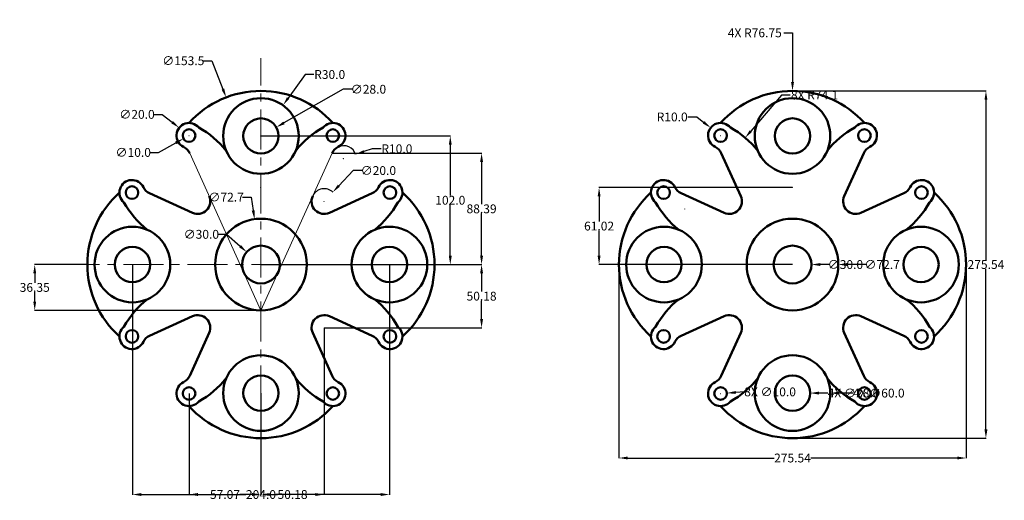
# Model space of a CAD drawing. Units: millimetres. Extents: x -118 to 663, y -125 to 257.
import ezdxf

# ---------------------------------------------------------------- set-up
doc = ezdxf.new("R2010")
doc.units = ezdxf.units.MM
doc.header["$MEASUREMENT"] = 0
doc.linetypes.add('CENTER', pattern=[50.8, 31.75, -6.35, 6.35, -6.35])
for name, color, linetype, lineweight in [('M-CNTR', 1, 'CENTER', 18), ('M-CONS', 8, 'Continuous', 13), ('M-DIMS', 3, 'Continuous', 25), ('M-OUTL', 7, 'Continuous', 50)]:
    doc.layers.add(name, color=color, linetype=linetype, lineweight=lineweight)
doc.styles.get("Standard").update_dxf_attribs({"font": 'arial.ttf'})
doc.dimstyles.get("Standard").update_dxf_attribs({"dimtxt": 7, "dimasz": 7, "dimexe": 0.18, "dimexo": 0.0625, "dimgap": 0.09, "dimtad": 0, "dimtih": 1, "dimtoh": 1, "dimdec": 1, "dimzin": 0, "dimdsep": 46, "dimtxsty": 'Standard', "dimcen": 0.09, "dimadec": 0, "dimazin": 0, "dimtfac": 1, "dimtdec": 1, "dimtofl": 0, "dimtmove": 0, "dimatfit": 3, "dimfxl": 1, "dimtolj": 1, "dimtzin": 0, "dimarcsym": 0})

# ---------------------------------------------------------------- blocks, each defined once
blk = doc.blocks.new('*D1')
at = {"layer": 'Defpoints', "color": 0, "transparency": 16777216}
for p in [(73.13, 164.34), (223.4, 164.34), (73.13, 62.34)]:
    blk.add_point(p, dxfattribs=at)
at = {"layer": 'M-DIMS', "color": 0, "lineweight": -2, "transparency": 16777216}
for p, q in [((73.19, 164.34), (223.58, 164.34)), ((223.4, 157.34), (223.4, 117.01)), ((223.4, 69.34), (223.4, 109.68)), ((73.19, 62.34), (223.58, 62.34))]:
    blk.add_line(p, q, dxfattribs=at)
at = {"layer": 'M-DIMS', "color": 0, "transparency": 16777216}
for points in [[(222.24, 157.34), (224.57, 157.34), (223.4, 164.34)], [(222.24, 69.34), (224.57, 69.34), (223.4, 62.34)]]:
    blk.add_solid(points, dxfattribs=at)
at = {"layer": 'M-DIMS', "color": 0, "transparency": 16777216, "insert": (223.4, 113.34), "char_height": 7, "attachment_point": 5}
blk.add_mtext('\\A1;102.0', dxfattribs=at)
blk = doc.blocks.new('*D2')
at = {"layer": 'Defpoints', "color": 0, "transparency": 16777216}
for p in [(130.17, 119.79), (116.43, 105.25)]:
    blk.add_point(p, dxfattribs=at)
at = {"layer": 'M-DIMS', "color": 0, "lineweight": -2, "transparency": 16777216}
for p, q in [((146.36, 136.91), (134.98, 124.87)), ((153.36, 136.91), (146.36, 136.91)), ((123.21, 112.52), (123.39, 112.52)), ((123.3, 112.43), (123.3, 112.61))]:
    blk.add_line(p, q, dxfattribs=at)
blk.add_arc((123.3, 112.52), 10, 45.57695, 155.27019, dxfattribs=at)
at = {"layer": 'M-DIMS', "color": 0, "transparency": 16777216}
blk.add_solid([(134.14, 125.67), (135.83, 124.07), (130.17, 119.79)], dxfattribs=at)
at = {"layer": 'M-DIMS', "color": 0, "transparency": 16777216, "insert": (166.34, 136.91), "char_height": 7, "attachment_point": 5}
blk.add_mtext('\\A1;∅20.0', dxfattribs=at)
blk = doc.blocks.new('*D3')
at = {"layer": 'Defpoints', "color": 0, "transparency": 16777216}
for p in [(61.85, 72.23), (84.4, 52.45)]:
    blk.add_point(p, dxfattribs=at)
at = {"layer": 'M-DIMS', "color": 0, "lineweight": -2, "transparency": 16777216}
for p, q in [((38.8, 86.31), (45.8, 86.31)), ((45.8, 86.31), (56.59, 76.85)), ((73.04, 62.34), (73.22, 62.34)), ((73.13, 62.25), (73.13, 62.43))]:
    blk.add_line(p, q, dxfattribs=at)
at = {"layer": 'M-DIMS', "color": 0, "transparency": 16777216}
blk.add_solid([(57.36, 77.73), (55.82, 75.97), (61.85, 72.23)], dxfattribs=at)
at = {"layer": 'M-DIMS', "color": 0, "transparency": 16777216, "insert": (25.82, 86.31), "char_height": 7, "attachment_point": 5}
blk.add_mtext('\\A1;∅30.0', dxfattribs=at)
blk = doc.blocks.new('*D4')
at = {"layer": 'Defpoints', "color": 0, "transparency": 16777216}
for p in [(67.99, 98.33), (78.26, 26.36)]:
    blk.add_point(p, dxfattribs=at)
at = {"layer": 'M-DIMS', "color": 0, "lineweight": -2, "transparency": 16777216}
for p, q in [((58.49, 115.82), (65.49, 115.82)), ((65.49, 115.82), (67, 105.26)), ((73.04, 62.34), (73.22, 62.34)), ((73.13, 62.25), (73.13, 62.43))]:
    blk.add_line(p, q, dxfattribs=at)
at = {"layer": 'M-DIMS', "color": 0, "transparency": 16777216}
blk.add_solid([(68.16, 105.42), (65.85, 105.09), (67.99, 98.33)], dxfattribs=at)
at = {"layer": 'M-DIMS', "color": 0, "transparency": 16777216, "insert": (45.5, 115.82), "char_height": 7, "attachment_point": 5}
blk.add_mtext('\\A1;∅72.7', dxfattribs=at)
blk = doc.blocks.new('*D5')
at = {"layer": 'Defpoints', "color": 0, "transparency": 16777216}
for p in [(20.44, 167.09), (11.68, 162.27)]:
    blk.add_point(p, dxfattribs=at)
at = {"layer": 'M-DIMS', "color": 0, "lineweight": -2, "transparency": 16777216}
for p, q in [((15.97, 164.68), (16.15, 164.68)), ((16.06, 164.59), (16.06, 164.77)), ((-8.28, 151.29), (5.54, 158.9)), ((-15.28, 151.29), (-8.28, 151.29))]:
    blk.add_line(p, q, dxfattribs=at)
at = {"layer": 'M-DIMS', "color": 0, "transparency": 16777216}
blk.add_solid([(4.98, 159.92), (6.11, 157.88), (11.68, 162.27)], dxfattribs=at)
at = {"layer": 'M-DIMS', "color": 0, "transparency": 16777216, "insert": (-28.26, 151.29), "char_height": 7, "attachment_point": 5}
blk.add_mtext('\\A1;∅10.0', dxfattribs=at)
blk = doc.blocks.new('*D6')
at = {"layer": 'Defpoints', "color": 0, "transparency": 16777216}
for p in [(8.21, 170.87), (23.91, 158.49)]:
    blk.add_point(p, dxfattribs=at)
at = {"layer": 'M-DIMS', "color": 0, "lineweight": -2, "transparency": 16777216}
for p, q in [((-12.26, 181.48), (-5.26, 181.48)), ((-5.26, 181.48), (2.71, 175.2)), ((15.97, 164.68), (16.15, 164.68)), ((16.06, 164.59), (16.06, 164.77))]:
    blk.add_line(p, q, dxfattribs=at)
at = {"layer": 'M-DIMS', "color": 0, "transparency": 16777216}
blk.add_solid([(3.43, 176.12), (1.99, 174.29), (8.21, 170.87)], dxfattribs=at)
at = {"layer": 'M-DIMS', "color": 0, "transparency": 16777216, "insert": (-25.24, 181.48), "char_height": 7, "attachment_point": 5}
blk.add_mtext('\\A1;∅20.0', dxfattribs=at)
blk = doc.blocks.new('*D7')
at = {"layer": 'Defpoints', "color": 0, "transparency": 16777216}
for p in [(85.3, 171.25), (60.95, 157.44)]:
    blk.add_point(p, dxfattribs=at)
at = {"layer": 'M-DIMS', "color": 0, "lineweight": -2, "transparency": 16777216}
for p, q in [((138.48, 201.41), (91.39, 174.7)), ((145.48, 201.41), (138.48, 201.41)), ((73.04, 164.34), (73.22, 164.34)), ((73.13, 164.25), (73.13, 164.43))]:
    blk.add_line(p, q, dxfattribs=at)
at = {"layer": 'M-DIMS', "color": 0, "transparency": 16777216}
blk.add_solid([(90.82, 175.72), (91.97, 173.69), (85.3, 171.25)], dxfattribs=at)
at = {"layer": 'M-DIMS', "color": 0, "transparency": 16777216, "insert": (158.46, 201.41), "char_height": 7, "attachment_point": 5}
blk.add_mtext('\\A1;∅28.0', dxfattribs=at)
blk = doc.blocks.new('*D8')
at = {"layer": 'Defpoints', "color": 0, "transparency": 16777216}
for p in [(90.64, 188.7), (73.13, 164.34)]:
    blk.add_point(p, dxfattribs=at)
at = {"layer": 'M-DIMS', "color": 0, "lineweight": -2, "transparency": 16777216}
for p, q in [((108.18, 213.12), (94.72, 194.39)), ((115.18, 213.12), (108.18, 213.12)), ((73.04, 164.34), (73.22, 164.34)), ((73.13, 164.25), (73.13, 164.43))]:
    blk.add_line(p, q, dxfattribs=at)
at = {"layer": 'M-DIMS', "color": 0, "transparency": 16777216}
blk.add_solid([(93.77, 195.07), (95.67, 193.71), (90.64, 188.7)], dxfattribs=at)
at = {"layer": 'M-DIMS', "color": 0, "transparency": 16777216, "insert": (127.7, 213.12), "char_height": 7, "attachment_point": 5}
blk.add_mtext('\\A1;R30.0', dxfattribs=at)
blk = doc.blocks.new('*D9')
at = {"layer": 'Defpoints', "color": 0, "transparency": 16777216}
for p in [(148.23, 149.76), (138.74, 146.6)]:
    blk.add_point(p, dxfattribs=at)
at = {"layer": 'M-DIMS', "color": 0, "lineweight": -2, "transparency": 16777216}
for p, q in [((161.51, 154.19), (154.87, 151.97)), ((168.51, 154.19), (161.51, 154.19)), ((138.65, 146.6), (138.83, 146.6)), ((138.74, 146.51), (138.74, 146.69))]:
    blk.add_line(p, q, dxfattribs=at)
blk.add_arc((138.74, 146.6), 10, 17.39119, 114.94899, dxfattribs=at)
at = {"layer": 'M-DIMS', "color": 0, "transparency": 16777216}
blk.add_solid([(154.5, 153.08), (155.24, 150.87), (148.23, 149.76)], dxfattribs=at)
at = {"layer": 'M-DIMS', "color": 0, "transparency": 16777216, "insert": (181.03, 154.19), "char_height": 7, "attachment_point": 5}
blk.add_mtext('\\A1;R10.0', dxfattribs=at)
blk = doc.blocks.new('*D10')
at = {"layer": 'Defpoints', "color": 0, "transparency": 16777216}
for p in [(45.48, 194.96), (100.77, 51.76)]:
    blk.add_point(p, dxfattribs=at)
at = {"layer": 'M-DIMS', "color": 0, "lineweight": -2, "transparency": 16777216}
for p, q in [((27.25, 224.05), (34.25, 224.05)), ((34.25, 224.05), (42.96, 201.49)), ((73.04, 123.36), (73.22, 123.36)), ((73.13, 123.27), (73.13, 123.45))]:
    blk.add_line(p, q, dxfattribs=at)
at = {"layer": 'M-DIMS', "color": 0, "transparency": 16777216}
blk.add_solid([(44.05, 201.91), (41.87, 201.07), (45.48, 194.96)], dxfattribs=at)
at = {"layer": 'M-DIMS', "color": 0, "transparency": 16777216, "insert": (11.51, 224.05), "char_height": 7, "attachment_point": 5}
blk.add_mtext('\\A1;∅153.5', dxfattribs=at)
blk = doc.blocks.new('*D11')
at = {"layer": 'Defpoints', "color": 0, "transparency": 16777216}
for p in [(-28.87, 62.34), (175.13, 62.34), (175.13, -120.14)]:
    blk.add_point(p, dxfattribs=at)
at = {"layer": 'M-DIMS', "color": 0, "lineweight": -2, "transparency": 16777216}
for p, q in [((-28.87, 62.28), (-28.87, -120.32)), ((175.13, 62.28), (175.13, -120.32)), ((-21.87, -120.14), (61.18, -120.14)), ((168.13, -120.14), (85.08, -120.14))]:
    blk.add_line(p, q, dxfattribs=at)
at = {"layer": 'M-DIMS', "color": 0, "transparency": 16777216}
for points in [[(-21.87, -118.97), (-21.87, -121.3), (-28.87, -120.14)], [(168.13, -118.97), (168.13, -121.3), (175.13, -120.14)]]:
    blk.add_solid(points, dxfattribs=at)
at = {"layer": 'M-DIMS', "color": 0, "transparency": 16777216, "insert": (73.13, -120.14), "char_height": 7, "attachment_point": 5}
blk.add_mtext('\\A1;204.0', dxfattribs=at)
blk = doc.blocks.new('*D12')
at = {"layer": 'Defpoints', "color": 0, "transparency": 16777216}
for p in [(16.06, -40), (73.13, -39.66), (73.13, -120.14)]:
    blk.add_point(p, dxfattribs=at)
at = {"layer": 'M-DIMS', "color": 0, "lineweight": -2, "transparency": 16777216}
for p, q in [((16.06, -40.06), (16.06, -120.32)), ((73.13, -39.72), (73.13, -120.32)), ((23.06, -120.14), (32.69, -120.14)), ((66.13, -120.14), (56.49, -120.14))]:
    blk.add_line(p, q, dxfattribs=at)
at = {"layer": 'M-DIMS', "color": 0, "transparency": 16777216}
for points in [[(23.06, -118.97), (23.06, -121.3), (16.06, -120.14)], [(66.13, -118.97), (66.13, -121.3), (73.13, -120.14)]]:
    blk.add_solid(points, dxfattribs=at)
at = {"layer": 'M-DIMS', "color": 0, "transparency": 16777216, "insert": (44.59, -120.14), "char_height": 7, "attachment_point": 5}
blk.add_mtext('\\A1;57.07', dxfattribs=at)
blk = doc.blocks.new('*D13')
at = {"layer": 'Defpoints', "color": 0, "transparency": 16777216}
for p in [(357.26, 62.34), (632.8, 62.34), (632.8, -91.18)]:
    blk.add_point(p, dxfattribs=at)
at = {"layer": 'M-DIMS', "color": 0, "lineweight": -2, "transparency": 16777216}
for p, q in [((357.26, 62.28), (357.26, -91.36)), ((632.8, 62.28), (632.8, -91.36)), ((364.26, -91.18), (480.37, -91.18)), ((625.8, -91.18), (509.7, -91.18))]:
    blk.add_line(p, q, dxfattribs=at)
at = {"layer": 'M-DIMS', "color": 0, "transparency": 16777216}
for points in [[(364.26, -90.01), (364.26, -92.34), (357.26, -91.18)], [(625.8, -90.01), (625.8, -92.34), (632.8, -91.18)]]:
    blk.add_solid(points, dxfattribs=at)
at = {"layer": 'M-DIMS', "color": 0, "transparency": 16777216, "insert": (495.03, -91.18), "char_height": 7, "attachment_point": 5}
blk.add_mtext('\\A1;275.54', dxfattribs=at)
blk = doc.blocks.new('*D14')
at = {"layer": 'Defpoints', "color": 0, "transparency": 16777216}
for p in [(495.03, 200.11), (495.03, -75.43), (648.55, -75.43)]:
    blk.add_point(p, dxfattribs=at)
at = {"layer": 'M-DIMS', "color": 0, "lineweight": -2, "transparency": 16777216}
for p, q in [((495.09, 200.11), (648.73, 200.11)), ((648.55, 193.11), (648.55, 66.01)), ((648.55, -68.43), (648.55, 58.68)), ((495.09, -75.43), (648.73, -75.43))]:
    blk.add_line(p, q, dxfattribs=at)
at = {"layer": 'M-DIMS', "color": 0, "transparency": 16777216}
for points in [[(647.38, 193.11), (649.72, 193.11), (648.55, 200.11)], [(647.38, -68.43), (649.72, -68.43), (648.55, -75.43)]]:
    blk.add_solid(points, dxfattribs=at)
at = {"layer": 'M-DIMS', "color": 0, "transparency": 16777216, "insert": (648.55, 62.34), "char_height": 7, "attachment_point": 5}
blk.add_mtext('\\A1;275.54', dxfattribs=at)
blk = doc.blocks.new('*D15')
at = {"layer": 'Defpoints', "color": 0, "transparency": 16777216}
for p in [(-64.64, 62.34), (-106.42, 25.99), (73.13, 25.99)]:
    blk.add_point(p, dxfattribs=at)
at = {"layer": 'M-DIMS', "color": 0, "lineweight": -2, "transparency": 16777216}
for p, q in [((-64.7, 62.34), (-106.6, 62.34)), ((-106.42, 55.34), (-106.42, 47.83)), ((-106.42, 32.99), (-106.42, 40.5)), ((73.06, 25.99), (-106.6, 25.99))]:
    blk.add_line(p, q, dxfattribs=at)
at = {"layer": 'M-DIMS', "color": 0, "transparency": 16777216}
for points in [[(-107.58, 55.34), (-105.25, 55.34), (-106.42, 62.34)], [(-107.58, 32.99), (-105.25, 32.99), (-106.42, 25.99)]]:
    blk.add_solid(points, dxfattribs=at)
at = {"layer": 'M-DIMS', "color": 0, "transparency": 16777216, "insert": (-106.42, 44.17), "char_height": 7, "attachment_point": 5}
blk.add_mtext('\\A1;36.35', dxfattribs=at)
blk = doc.blocks.new('*D16')
at = {"layer": 'Defpoints', "color": 0, "transparency": 16777216}
for p in [(341.51, 123.36), (495.03, 123.36), (495.03, 62.34)]:
    blk.add_point(p, dxfattribs=at)
at = {"layer": 'M-DIMS', "color": 0, "lineweight": -2, "transparency": 16777216}
for p, q in [((494.97, 123.36), (341.33, 123.36)), ((341.51, 116.36), (341.51, 96.52)), ((341.51, 69.34), (341.51, 89.19)), ((494.97, 62.34), (341.33, 62.34))]:
    blk.add_line(p, q, dxfattribs=at)
at = {"layer": 'M-DIMS', "color": 0, "transparency": 16777216}
for points in [[(340.35, 116.36), (342.68, 116.36), (341.51, 123.36)], [(340.35, 69.34), (342.68, 69.34), (341.51, 62.34)]]:
    blk.add_solid(points, dxfattribs=at)
at = {"layer": 'M-DIMS', "color": 0, "transparency": 16777216, "insert": (341.51, 92.85), "char_height": 7, "attachment_point": 5}
blk.add_mtext('\\A1;61.02', dxfattribs=at)
blk = doc.blocks.new('*D17')
at = {"layer": 'Defpoints', "color": 0, "transparency": 16777216}
for p in [(129.63, 150.73), (248.25, 150.73), (175.13, 62.34)]:
    blk.add_point(p, dxfattribs=at)
at = {"layer": 'M-DIMS', "color": 0, "lineweight": -2, "transparency": 16777216}
for p, q in [((129.7, 150.73), (248.43, 150.73)), ((248.25, 143.73), (248.25, 110.2)), ((248.25, 69.34), (248.25, 102.87)), ((175.19, 62.34), (248.43, 62.34))]:
    blk.add_line(p, q, dxfattribs=at)
at = {"layer": 'M-DIMS', "color": 0, "transparency": 16777216}
for points in [[(247.08, 143.73), (249.41, 143.73), (248.25, 150.73)], [(247.08, 69.34), (249.41, 69.34), (248.25, 62.34)]]:
    blk.add_solid(points, dxfattribs=at)
at = {"layer": 'M-DIMS', "color": 0, "transparency": 16777216, "insert": (248.25, 106.53), "char_height": 7, "attachment_point": 5}
blk.add_mtext('\\A1;88.39', dxfattribs=at)
blk = doc.blocks.new('*D18')
at = {"layer": 'Defpoints', "color": 0, "transparency": 16777216}
for p in [(123.3, 12.16), (73.13, -39.66), (123.3, -120.14)]:
    blk.add_point(p, dxfattribs=at)
at = {"layer": 'M-DIMS', "color": 0, "lineweight": -2, "transparency": 16777216}
for p, q in [((123.3, 12.1), (123.3, -120.32)), ((73.13, -39.72), (73.13, -120.32)), ((80.13, -120.14), (86.31, -120.14)), ((116.3, -120.14), (110.12, -120.14))]:
    blk.add_line(p, q, dxfattribs=at)
at = {"layer": 'M-DIMS', "color": 0, "transparency": 16777216}
for points in [[(80.13, -118.97), (80.13, -121.3), (73.13, -120.14)], [(116.3, -118.97), (116.3, -121.3), (123.3, -120.14)]]:
    blk.add_solid(points, dxfattribs=at)
at = {"layer": 'M-DIMS', "color": 0, "transparency": 16777216, "insert": (98.22, -120.14), "char_height": 7, "attachment_point": 5}
blk.add_mtext('\\A1;50.18', dxfattribs=at)
blk = doc.blocks.new('*D19')
at = {"layer": 'Defpoints', "color": 0, "transparency": 16777216}
for p in [(175.13, 62.34), (123.3, 12.16), (248.25, 12.16)]:
    blk.add_point(p, dxfattribs=at)
at = {"layer": 'M-DIMS', "color": 0, "lineweight": -2, "transparency": 16777216}
for p, q in [((175.19, 62.34), (248.43, 62.34)), ((248.25, 55.34), (248.25, 40.92)), ((248.25, 19.16), (248.25, 33.59)), ((123.37, 12.16), (248.43, 12.16))]:
    blk.add_line(p, q, dxfattribs=at)
at = {"layer": 'M-DIMS', "color": 0, "transparency": 16777216}
for points in [[(247.08, 55.34), (249.41, 55.34), (248.25, 62.34)], [(247.08, 19.16), (249.41, 19.16), (248.25, 12.16)]]:
    blk.add_solid(points, dxfattribs=at)
at = {"layer": 'M-DIMS', "color": 0, "transparency": 16777216, "insert": (248.25, 37.25), "char_height": 7, "attachment_point": 5}
blk.add_mtext('\\A1;50.18', dxfattribs=at)
blk = doc.blocks.new('*D20')
at = {"layer": 'Defpoints', "color": 0, "transparency": 16777216}
for p in [(495.03, 200.11), (495.03, 123.36)]:
    blk.add_point(p, dxfattribs=at)
at = {"layer": 'M-DIMS', "color": 0, "lineweight": -2, "transparency": 16777216}
for p, q in [((488.02, 246.16), (495.02, 246.16)), ((495.02, 246.16), (495.03, 207.11)), ((494.94, 123.36), (495.12, 123.36)), ((495.03, 123.27), (495.03, 123.45))]:
    blk.add_line(p, q, dxfattribs=at)
at = {"layer": 'M-DIMS', "color": 0, "transparency": 16777216}
blk.add_solid([(496.19, 207.11), (493.86, 207.11), (495.03, 200.11)], dxfattribs=at)
at = {"layer": 'M-DIMS', "color": 0, "transparency": 16777216, "insert": (465.09, 246.16), "char_height": 7, "attachment_point": 5}
blk.add_mtext('\\A1;4X R76.75', dxfattribs=at)
blk = doc.blocks.new('*D21')
at = {"layer": 'Defpoints', "color": 0, "transparency": 16777216}
for p in [(457.44, 162.89), (409.54, 106.34)]:
    blk.add_point(p, dxfattribs=at)
at = {"layer": 'M-DIMS', "color": 0, "lineweight": -2, "transparency": 16777216}
for p, q in [((486.18, 196.82), (461.96, 168.23)), ((493.18, 196.82), (486.18, 196.82)), ((409.45, 106.34), (409.63, 106.34)), ((409.54, 106.25), (409.54, 106.43))]:
    blk.add_line(p, q, dxfattribs=at)
at = {"layer": 'M-DIMS', "color": 0, "transparency": 16777216}
blk.add_solid([(461.07, 168.98), (462.85, 167.47), (457.44, 162.89)], dxfattribs=at)
at = {"layer": 'M-DIMS', "color": 0, "transparency": 16777216, "insert": (512.56, 196.82), "char_height": 7, "attachment_point": 5}
blk.add_mtext('\\A1;8X R74.1', dxfattribs=at)
blk = doc.blocks.new('*D22')
at = {"layer": 'Defpoints', "color": 0, "transparency": 16777216}
for p in [(458.68, 62.34), (531.38, 62.34)]:
    blk.add_point(p, dxfattribs=at)
at = {"layer": 'M-DIMS', "color": 0, "lineweight": -2, "transparency": 16777216}
for p, q in [((494.94, 62.34), (495.12, 62.34)), ((495.03, 62.25), (495.03, 62.43)), ((553.19, 62.34), (538.38, 62.34))]:
    blk.add_line(p, q, dxfattribs=at)
at = {"layer": 'M-DIMS', "color": 0, "transparency": 16777216}
blk.add_solid([(538.38, 63.51), (538.38, 61.18), (531.38, 62.34)], dxfattribs=at)
at = {"layer": 'M-DIMS', "color": 0, "transparency": 16777216, "insert": (566.18, 62.34), "char_height": 7, "attachment_point": 5}
blk.add_mtext('\\A1;∅72.7', dxfattribs=at)
blk = doc.blocks.new('*D23')
at = {"layer": 'Defpoints', "color": 0, "transparency": 16777216}
for p in [(480.03, 62.34), (510.03, 62.34)]:
    blk.add_point(p, dxfattribs=at)
at = {"layer": 'M-DIMS', "color": 0, "lineweight": -2, "transparency": 16777216}
for p, q in [((494.94, 62.34), (495.12, 62.34)), ((495.03, 62.25), (495.03, 62.43)), ((524.03, 62.34), (517.03, 62.34))]:
    blk.add_line(p, q, dxfattribs=at)
at = {"layer": 'M-DIMS', "color": 0, "transparency": 16777216}
blk.add_solid([(517.03, 63.51), (517.03, 61.18), (510.03, 62.34)], dxfattribs=at)
at = {"layer": 'M-DIMS', "color": 0, "transparency": 16777216, "insert": (537.01, 62.34), "char_height": 7, "attachment_point": 5}
blk.add_mtext('\\A1;∅30.0', dxfattribs=at)
blk = doc.blocks.new('*D24')
at = {"layer": 'Defpoints', "color": 0, "transparency": 16777216}
for p in [(465.03, -39.66), (525.03, -39.66)]:
    blk.add_point(p, dxfattribs=at)
at = {"layer": 'M-DIMS', "color": 0, "lineweight": -2, "transparency": 16777216}
for p, q in [((494.94, -39.66), (495.12, -39.66)), ((495.03, -39.75), (495.03, -39.57)), ((543.03, -39.66), (532.03, -39.66))]:
    blk.add_line(p, q, dxfattribs=at)
at = {"layer": 'M-DIMS', "color": 0, "transparency": 16777216}
blk.add_solid([(532.03, -38.49), (532.03, -40.82), (525.03, -39.66)], dxfattribs=at)
at = {"layer": 'M-DIMS', "color": 0, "transparency": 16777216, "insert": (563.48, -39.66), "char_height": 7, "attachment_point": 5}
blk.add_mtext('\\A1;4X ∅60.0', dxfattribs=at)
blk = doc.blocks.new('*D25')
at = {"layer": 'Defpoints', "color": 0, "transparency": 16777216}
for p in [(481.03, -39.66), (509.03, -39.66)]:
    blk.add_point(p, dxfattribs=at)
at = {"layer": 'M-DIMS', "color": 0, "lineweight": -2, "transparency": 16777216}
for p, q in [((494.94, -39.66), (495.12, -39.66)), ((495.03, -39.75), (495.03, -39.57)), ((523.03, -39.66), (516.03, -39.66))]:
    blk.add_line(p, q, dxfattribs=at)
at = {"layer": 'M-DIMS', "color": 0, "transparency": 16777216}
blk.add_solid([(516.03, -38.49), (516.03, -40.82), (509.03, -39.66)], dxfattribs=at)
at = {"layer": 'M-DIMS', "color": 0, "transparency": 16777216, "insert": (543.48, -39.66), "char_height": 7, "attachment_point": 5}
blk.add_mtext('\\A1;4X ∅28.0', dxfattribs=at)
blk = doc.blocks.new('*D26')
at = {"layer": 'Defpoints', "color": 0, "transparency": 16777216}
for p in [(432.97, -40.34), (442.95, -39.65)]:
    blk.add_point(p, dxfattribs=at)
at = {"layer": 'M-DIMS', "color": 0, "lineweight": -2, "transparency": 16777216}
for p, q in [((456.92, -38.7), (449.93, -39.18)), ((437.87, -40), (438.05, -40)), ((437.96, -40.09), (437.96, -39.91))]:
    blk.add_line(p, q, dxfattribs=at)
at = {"layer": 'M-DIMS', "color": 0, "transparency": 16777216}
blk.add_solid([(449.85, -38.01), (450.01, -40.34), (442.95, -39.65)], dxfattribs=at)
at = {"layer": 'M-DIMS', "color": 0, "transparency": 16777216, "insert": (477.23, -38.7), "char_height": 7, "attachment_point": 5}
blk.add_mtext('\\A1;8X ∅10.0', dxfattribs=at)
blk = doc.blocks.new('*D27')
at = {"layer": 'Defpoints', "color": 0, "transparency": 16777216}
for p in [(430.07, 170.83), (437.96, 164.68)]:
    blk.add_point(p, dxfattribs=at)
at = {"layer": 'M-DIMS', "color": 0, "lineweight": -2, "transparency": 16777216}
for p, q in [((412.03, 179.43), (419.03, 179.43)), ((419.03, 179.43), (424.55, 175.13)), ((437.87, 164.68), (438.05, 164.68)), ((437.96, 164.59), (437.96, 164.77))]:
    blk.add_line(p, q, dxfattribs=at)
at = {"layer": 'M-DIMS', "color": 0, "transparency": 16777216}
blk.add_solid([(425.27, 176.05), (423.84, 174.21), (430.07, 170.83)], dxfattribs=at)
at = {"layer": 'M-DIMS', "color": 0, "transparency": 16777216, "insert": (399.51, 179.43), "char_height": 7, "attachment_point": 5}
blk.add_mtext('\\A1;R10.0', dxfattribs=at)

msp = doc.modelspace()

# ---------------------------------------------------------------- linework, layer by layer
at = {"layer": 'M-CNTR'}
for p, q in [((73.127, -100.386), (73.127, 225.978)), ((-86.667, 62.342), (228.498, 62.342))]:
    msp.add_line(p, q, dxfattribs=at)
at = {"layer": 'M-CONS'}
for q in [(16.619, 150.727), (129.635, 150.727)]:
    msp.add_line((73.127, 25.992), q, dxfattribs=at)
at = {"layer": 'M-OUTL'}
for p, q in [((453.962, 116.646), (438.522, 150.727)), ((536.099, 116.646), (551.539, 150.727)), ((18.823, 103.411), (-15.258, 118.85)), ((127.431, 103.411), (161.512, 118.85)), ((440.727, 103.411), (406.646, 118.85)), ((549.334, 103.411), (583.416, 118.85)), ((18.823, 21.274), (-15.258, 5.834)), ((127.431, 21.274), (161.512, 5.834)), ((440.727, 21.274), (406.646, 5.834)), ((549.334, 21.274), (583.416, 5.834)), ((32.058, 8.038), (16.619, -26.043)), ((114.195, 8.038), (129.635, -26.043)), ((453.962, 8.038), (438.522, -26.043)), ((536.099, 8.038), (551.539, -26.043))]:
    msp.add_line(p, q, dxfattribs=at)
for centre, radius in [((73.127, 164.342), 30), ((495.031, 164.342), 30), ((73.127, 164.342), 14), ((495.031, 164.342), 14), ((16.059, 164.681), 5), ((130.194, 164.681), 5), ((437.963, 164.681), 5), ((552.098, 164.681), 5), ((-29.212, 119.41), 5), ((175.466, 119.41), 5), ((392.691, 119.41), 5), ((597.37, 119.41), 5), ((73.127, 62.342), 36.35), ((495.031, 62.342), 36.35), ((-28.873, 62.342), 30), ((175.127, 62.342), 30), ((393.031, 62.342), 30), ((597.031, 62.342), 30), ((-28.873, 62.342), 14), ((73.127, 62.342), 15), ((175.127, 62.342), 14), ((393.031, 62.342), 14), ((495.031, 62.342), 15), ((597.031, 62.342), 14), ((-29.212, 5.275), 5), ((175.466, 5.275), 5), ((392.691, 5.275), 5), ((597.37, 5.275), 5), ((73.127, -39.658), 30), ((495.031, -39.658), 30), ((73.127, -39.658), 14), ((495.031, -39.658), 14), ((16.059, -39.997), 5), ((130.194, -39.997), 5), ((437.963, -39.997), 5), ((552.098, -39.997), 5)]:
    msp.add_circle(centre, radius, dxfattribs=at)
for centre, radius, start, end in [((73.127, 123.36), 76.75, 41.965163, 138.034837), ((495.031, 123.36), 76.75, 41.965163, 138.034837), ((16.059, 164.681), 10, 39.432865, 244.69291), ((130.194, 164.681), 10, 295.30709, 140.567135), ((437.963, 164.681), 10, 39.432865, 244.69291), ((552.098, 164.681), 10, 295.30709, 140.567135), ((-12.362, 106.338), 74.107, 38.658013, 60.807644), ((158.616, 106.338), 74.107, 119.192356, 141.341987), ((409.541, 106.338), 74.107, 38.658013, 60.807644), ((580.52, 106.338), 74.107, 119.192356, 141.341987), ((7.51, 146.601), 10, 24.371711, 64.69291), ((138.744, 146.601), 10, 115.30709, 155.628289), ((429.414, 146.601), 10, 24.371711, 64.69291), ((560.648, 146.601), 10, 115.30709, 155.628289), ((-29.212, 119.41), 10, 25.30709, 230.567135), ((175.466, 119.41), 10, 309.432865, 154.69291), ((392.691, 119.41), 10, 25.30709, 230.567135), ((597.37, 119.41), 10, 309.432865, 154.69291), ((12.109, 62.342), 76.75, 131.965163, 228.034837), ((-11.132, 127.959), 10, 205.30709, 245.628289), ((157.385, 127.959), 10, 294.371711, 334.69291), ((134.145, 62.342), 76.75, 311.965163, 48.034837), ((434.013, 62.342), 76.75, 131.965163, 228.034837), ((410.772, 127.959), 10, 205.30709, 245.628289), ((579.289, 127.959), 10, 294.371711, 334.69291), ((556.049, 62.342), 76.75, 311.965163, 48.034837), ((29.131, 147.831), 74.107, 209.192356, 231.341987), ((22.949, 112.52), 10, 245.628289, 24.371711), ((123.304, 112.52), 10, 155.628289, 294.371711), ((117.123, 147.831), 74.107, 308.658013, 330.807644), ((451.034, 147.831), 74.107, 209.192356, 231.341987), ((444.853, 112.52), 10, 245.628289, 24.371711), ((545.208, 112.52), 10, 155.628289, 294.371711), ((539.027, 147.831), 74.107, 308.658013, 330.807644), ((29.131, -23.147), 74.107, 128.658013, 150.807644), ((117.123, -23.147), 74.107, 29.192356, 51.341987), ((451.034, -23.147), 74.107, 128.658013, 150.807644), ((539.027, -23.147), 74.107, 29.192356, 51.341987), ((22.949, 12.165), 10, 335.628289, 114.371711), ((123.304, 12.165), 10, 65.628289, 204.371711), ((444.853, 12.165), 10, 335.628289, 114.371711), ((545.208, 12.165), 10, 65.628289, 204.371711), ((-29.212, 5.275), 10, 129.432865, 334.69291), ((175.466, 5.275), 10, 205.30709, 50.567135), ((392.691, 5.275), 10, 129.432865, 334.69291), ((597.37, 5.275), 10, 205.30709, 50.567135), ((-11.132, -3.275), 10, 114.371711, 154.69291), ((157.385, -3.275), 10, 25.30709, 65.628289), ((410.772, -3.275), 10, 114.371711, 154.69291), ((579.289, -3.275), 10, 25.30709, 65.628289), ((16.059, -39.997), 10, 115.30709, 320.567135), ((7.51, -21.916), 10, 295.30709, 335.628289), ((-12.362, 18.346), 74.107, 299.192356, 321.341987), ((158.616, 18.346), 74.107, 218.658013, 240.807644), ((130.194, -39.997), 10, 219.432865, 64.69291), ((138.744, -21.916), 10, 204.371711, 244.69291), ((437.963, -39.997), 10, 115.30709, 320.567135), ((429.414, -21.916), 10, 295.30709, 335.628289), ((409.541, 18.346), 74.107, 299.192356, 321.341987), ((580.52, 18.346), 74.107, 218.658013, 240.807644), ((552.098, -39.997), 10, 219.432865, 64.69291), ((560.648, -21.916), 10, 204.371711, 244.69291), ((73.127, 1.324), 76.75, 221.965163, 318.034837), ((495.031, 1.324), 76.75, 221.965163, 318.034837)]:
    msp.add_arc(centre, radius, start, end, dxfattribs=at)

# ---------------------------------------------------------------- dimensions: what is measured, and where the dimension line sits
at = {"layer": 'M-DIMS'}
for center, mpoint, text, override, picture, middle in [((495.031, 123.36), (495.027, 200.11), '4X <>', {"dimdec": 2, "dimlfac": 1, "dimrnd": 0, "dimzin": 0, "dimdsep": 46, "dimlunit": 2}, '*D20', (465.087, 246.16)), ((409.541, 106.338), (457.439, 162.887), '8X <>', {"dimdec": 1, "dimlfac": 1, "dimrnd": 0, "dimzin": 0, "dimdsep": 46, "dimlunit": 2}, '*D21', (512.558, 196.816))]:
    dim = msp.add_radius_dim(center=center, mpoint=mpoint, text=text, dimstyle='Standard', override=override, dxfattribs=at)
    dim.commit()
    dim.dimension.update_dxf_attribs({"geometry": picture, "text_midpoint": middle, "dimtype": 164})
for p1, p2, override, picture, middle in [((100.772, 51.762), (45.481, 194.958), {"dimclrd": 0, "dimclre": 0, "dimclrt": 0}, '*D10', (11.512, 224.054)), ((458.681, 62.342), (531.381, 62.342), {"dimdec": 1, "dimlfac": 1, "dimrnd": 0, "dimzin": 0, "dimdsep": 46, "dimlunit": 2}, '*D22', (553.191, 62.342)), ((480.031, 62.342), (510.031, 62.342), {"dimdec": 1, "dimlfac": 1, "dimrnd": 0, "dimzin": 0, "dimdsep": 46, "dimlunit": 2}, '*D23', (524.031, 62.342))]:
    dim = msp.add_diameter_dim_2p(p1=p1, p2=p2, dimstyle='Standard', override=override, dxfattribs=at)
    dim.commit()
    dim.dimension.update_dxf_attribs({"geometry": picture, "text_midpoint": middle, "dimtype": 163})
at = {"layer": 'M-DIMS', "transparency": 33554610}
dim = msp.add_radius_dim(center=(73.127, 164.342), mpoint=(90.635, 188.703), dimstyle='Standard', override={"dimclrd": 0, "dimclre": 0, "dimclrt": 0}, dxfattribs=at)
dim.commit()
dim.dimension.update_dxf_attribs({"geometry": '*D8', "text_midpoint": (127.699, 213.116), "dimtype": 164})
for p1, p2, picture, middle in [((60.949, 157.435), (85.304, 171.249), '*D7', (158.456, 201.41)), ((23.913, 158.491), (8.206, 170.872), '*D6', (-25.235, 181.483)), ((20.44, 167.091), (11.678, 162.272), '*D5', (-28.257, 151.294)), ((116.434, 105.253), (130.174, 119.786), '*D2', (166.341, 136.911)), ((78.263, 26.357), (67.991, 98.327), '*D4', (45.504, 115.82)), ((84.403, 52.451), (61.85, 72.234), '*D3', (25.823, 86.313))]:
    dim = msp.add_diameter_dim_2p(p1=p1, p2=p2, dimstyle='Standard', override={"dimclrd": 0, "dimclre": 0, "dimclrt": 0}, dxfattribs=at)
    dim.commit()
    dim.dimension.update_dxf_attribs({"geometry": picture, "text_midpoint": middle, "dimtype": 163})
at = {"layer": 'M-DIMS'}
for base, p1, p2, picture, middle in [((648.549, -75.426), (495.031, 200.11), (495.031, -75.426), '*D14', (648.549, 62.342)), ((248.2477, 150.7273), (175.1268, 62.3422), (129.6349, 150.7273), '*D17', (248.2477, 106.5347)), ((341.513, 123.36), (495.031, 62.342), (495.031, 123.36), '*D16', (341.513, 92.851)), ((-106.417, 25.992), (-64.641, 62.342), (73.127, 25.992), '*D15', (-106.417, 44.167)), ((248.248, 12.165), (175.127, 62.342), (123.304, 12.165), '*D19', (248.248, 37.254))]:
    dim = msp.add_linear_dim(base=base, p1=p1, p2=p2, angle=90, dimstyle='Standard', override={"dimdec": 2, "dimlfac": 1, "dimrnd": 0, "dimzin": 0, "dimdsep": 46, "dimlunit": 2}, dxfattribs=at)
    dim.commit()
    dim.dimension.update_dxf_attribs({"geometry": picture, "text_midpoint": middle})
dim = msp.add_radius_dim(center=(437.963, 164.681), mpoint=(430.074, 170.827), dimstyle='Standard', override={"dimdec": 1, "dimlfac": 1, "dimrnd": 0, "dimzin": 0, "dimdsep": 46, "dimlunit": 2}, dxfattribs=at)
dim.commit()
dim.dimension.update_dxf_attribs({"geometry": '*D27', "text_midpoint": (399.511, 179.431)})
at = {"layer": 'M-DIMS', "transparency": 33554610}
dim = msp.add_linear_dim(base=(223.404, 164.342), p1=(73.127, 62.342), p2=(73.127, 164.342), angle=90, dimstyle='Standard', override={"dimclrd": 0, "dimclre": 0, "dimclrt": 0}, dxfattribs=at)
dim.commit()
dim.dimension.update_dxf_attribs({"geometry": '*D1', "text_midpoint": (223.404, 113.342)})
dim = msp.add_radius_dim(center=(138.744, 146.601), mpoint=(148.231, 149.761), dimstyle='Standard', override={"dimclrd": 0, "dimclre": 0, "dimclrt": 0}, dxfattribs=at)
dim.commit()
dim.dimension.update_dxf_attribs({"geometry": '*D9', "text_midpoint": (181.033, 154.185)})
at = {"layer": 'M-DIMS'}
for base, p1, p2, override, picture, middle in [((175.127, -120.136), (-28.873, 62.342), (175.127, 62.342), {"dimdec": 1, "dimlfac": 1, "dimrnd": 0, "dimzin": 0, "dimdsep": 46, "dimlunit": 2}, '*D11', (73.127, -120.136)), ((632.799, -91.176), (357.263, 62.342), (632.799, 62.342), {"dimdec": 2, "dimlfac": 1, "dimrnd": 0, "dimzin": 0, "dimdsep": 46, "dimlunit": 2}, '*D13', (495.031, -91.176)), ((123.304, -120.136), (73.127, -39.658), (123.304, 12.165), {"dimdec": 2, "dimlfac": 1, "dimrnd": 0, "dimzin": 0, "dimdsep": 46, "dimlunit": 2}, '*D18', (98.216, -120.136)), ((73.127, -120.136), (16.059, -39.997), (73.127, -39.658), {"dimdec": 2, "dimlfac": 1, "dimrnd": 0, "dimzin": 0, "dimdsep": 46, "dimlunit": 2}, '*D12', (44.593, -120.136))]:
    dim = msp.add_linear_dim(base=base, p1=p1, p2=p2, dimstyle='Standard', override=override, dxfattribs=at)
    dim.commit()
    dim.dimension.update_dxf_attribs({"geometry": picture, "text_midpoint": middle})
for p1, p2, text, picture, middle in [((432.975, -40.339), (442.951, -39.654), '8X <>', '*D26', (456.918, -38.696)), ((465.031, -39.658), (525.031, -39.658), '4X <>', '*D24', (543.031, -39.658))]:
    dim = msp.add_diameter_dim_2p(p1=p1, p2=p2, text=text, dimstyle='Standard', override={"dimdec": 1, "dimlfac": 1, "dimrnd": 0, "dimzin": 0, "dimdsep": 46, "dimlunit": 2}, dxfattribs=at)
    dim.commit()
    dim.dimension.update_dxf_attribs({"geometry": picture, "text_midpoint": middle, "dimtype": 163})
dim = msp.add_diameter_dim_2p(p1=(481.031, -39.658), p2=(509.031, -39.658), text='4X <>', dimstyle='Standard', override={"dimdec": 1, "dimlfac": 1, "dimrnd": 0, "dimzin": 0, "dimdsep": 46, "dimlunit": 2}, dxfattribs=at)
dim.commit()
dim.dimension.update_dxf_attribs({"geometry": '*D25', "text_midpoint": (523.031, -39.658)})

doc.saveas('drawing.dxf')
